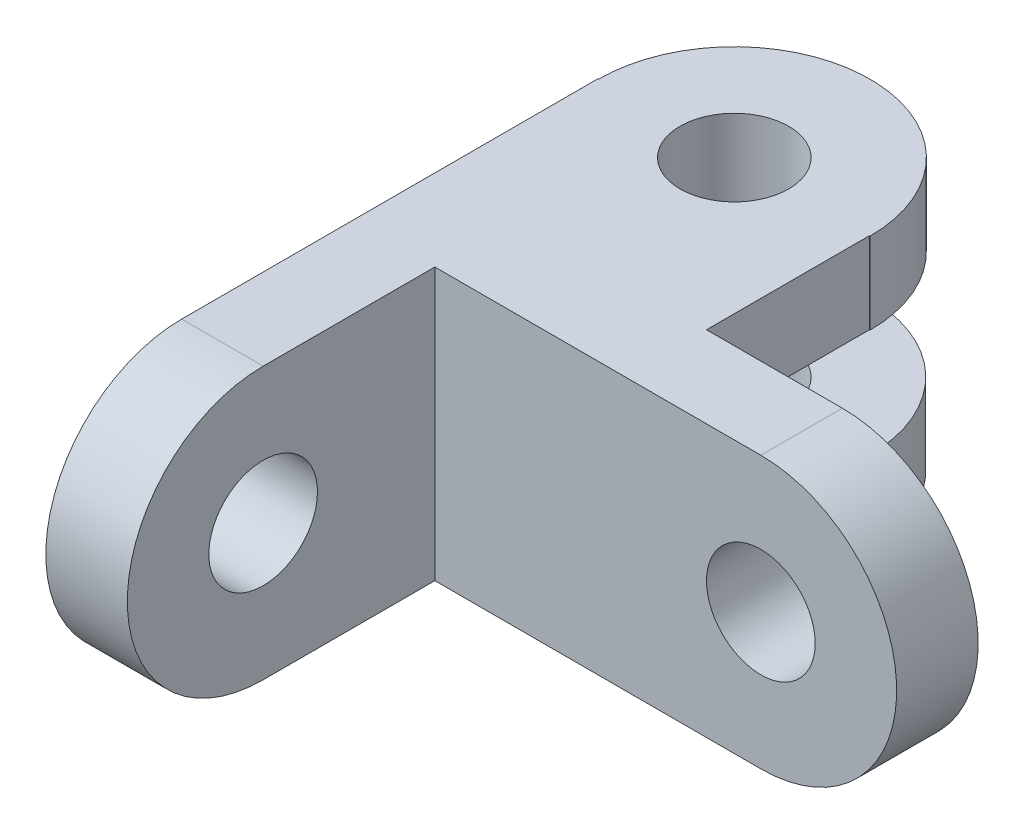
ISO-10303-21;
HEADER;
FILE_DESCRIPTION(('STEP AP214'),'2;1');
FILE_NAME('part.step','',(''),(''),'','','');
FILE_SCHEMA(('AUTOMOTIVE_DESIGN { 1 0 10303 214 1 1 1 1 }'));
ENDSEC;
DATA;
#1=APPLICATION_CONTEXT('core data for automotive mechanical design processes');
#2=APPLICATION_PROTOCOL_DEFINITION('international standard','automotive_design',2000,#1);
#3=PRODUCT_CONTEXT('',#1,'mechanical');
#4=PRODUCT('Part','Part','',(#3));
#5=PRODUCT_RELATED_PRODUCT_CATEGORY('part','',(#4));
#6=PRODUCT_DEFINITION_FORMATION('','',#4);
#7=PRODUCT_DEFINITION_CONTEXT('part definition',#1,'design');
#8=PRODUCT_DEFINITION('design','',#6,#7);
#9=PRODUCT_DEFINITION_SHAPE('','',#8);
#10=(LENGTH_UNIT() NAMED_UNIT(*) SI_UNIT(.MILLI.,.METRE.));
#11=(NAMED_UNIT(*) PLANE_ANGLE_UNIT() SI_UNIT($,.RADIAN.));
#12=(NAMED_UNIT(*) SI_UNIT($,.STERADIAN.) SOLID_ANGLE_UNIT());
#13=UNCERTAINTY_MEASURE_WITH_UNIT(LENGTH_MEASURE(1.E-05),#10,'distance_accuracy_value','');
#14=(GEOMETRIC_REPRESENTATION_CONTEXT(3) GLOBAL_UNCERTAINTY_ASSIGNED_CONTEXT((#13)) GLOBAL_UNIT_ASSIGNED_CONTEXT((#10,
#11,#12)) REPRESENTATION_CONTEXT('',''));
#15=CARTESIAN_POINT('',(0.,0.,0.));
#16=DIRECTION('',(0.,0.,1.));
#17=DIRECTION('',(1.,0.,0.));
#18=AXIS2_PLACEMENT_3D('',#15,#16,#17);
#19=CARTESIAN_POINT('',(0.,0.,6.));
#20=DIRECTION('',(0.,0.,1.));
#21=DIRECTION('',(1.,0.,0.));
#22=AXIS2_PLACEMENT_3D('',#19,#20,#21);
#23=PLANE('',#22);
#24=CARTESIAN_POINT('',(60.,20.,6.));
#25=DIRECTION('',(0.,0.,1.));
#26=DIRECTION('',(1.,0.,0.));
#27=AXIS2_PLACEMENT_3D('',#24,#25,#26);
#28=CIRCLE('',#27,8.00000000000001);
#29=CARTESIAN_POINT('',(68.,20.,6.));
#30=VERTEX_POINT('',#29);
#31=EDGE_CURVE('E519',#30,#30,#28,.T.);
#32=ORIENTED_EDGE('',*,*,#31,.F.);
#33=EDGE_LOOP('',(#32));
#34=FACE_BOUND('',#33,.T.);
#35=DIRECTION('',(1.,0.,0.));
#36=VECTOR('',#35,1.);
#37=CARTESIAN_POINT('',(0.,40.,6.));
#38=LINE('',#37,#36);
#39=CARTESIAN_POINT('',(12.,40.,6.));
#40=VERTEX_POINT('',#39);
#41=CARTESIAN_POINT('',(60.,40.,6.));
#42=VERTEX_POINT('',#41);
#43=EDGE_CURVE('E252',#40,#42,#38,.T.);
#44=ORIENTED_EDGE('',*,*,#43,.F.);
#45=DIRECTION('',(0.,-1.,0.));
#46=VECTOR('',#45,1.);
#47=CARTESIAN_POINT('',(12.,40.,6.));
#48=LINE('',#47,#46);
#49=CARTESIAN_POINT('',(12.,0.,6.));
#50=VERTEX_POINT('',#49);
#51=EDGE_CURVE('E161',#40,#50,#48,.T.);
#52=ORIENTED_EDGE('',*,*,#51,.T.);
#53=DIRECTION('',(1.,0.,0.));
#54=VECTOR('',#53,1.);
#55=CARTESIAN_POINT('',(0.,0.,6.));
#56=LINE('',#55,#54);
#57=CARTESIAN_POINT('',(60.,0.,6.));
#58=VERTEX_POINT('',#57);
#59=EDGE_CURVE('E162',#50,#58,#56,.T.);
#60=ORIENTED_EDGE('',*,*,#59,.T.);
#61=CARTESIAN_POINT('',(60.,20.,6.));
#62=DIRECTION('',(0.,0.,1.));
#63=DIRECTION('',(1.,0.,0.));
#64=AXIS2_PLACEMENT_3D('',#61,#62,#63);
#65=CIRCLE('',#64,20.);
#66=EDGE_CURVE('E250',#58,#42,#65,.T.);
#67=ORIENTED_EDGE('',*,*,#66,.T.);
#68=EDGE_LOOP('',(#44,#52,#60,#67));
#69=FACE_BOUND('',#68,.T.);
#70=ADVANCED_FACE('F41',(#34,#69),#23,.T.);
#71=CARTESIAN_POINT('',(0.,0.,-6.));
#72=DIRECTION('',(0.,0.,1.));
#73=DIRECTION('',(1.,0.,0.));
#74=AXIS2_PLACEMENT_3D('',#71,#72,#73);
#75=PLANE('',#74);
#76=CARTESIAN_POINT('',(60.,20.,-6.));
#77=DIRECTION('',(0.,0.,1.));
#78=DIRECTION('',(1.,0.,0.));
#79=AXIS2_PLACEMENT_3D('',#76,#77,#78);
#80=CIRCLE('',#79,8.00000000000001);
#81=CARTESIAN_POINT('',(68.,20.,-6.));
#82=VERTEX_POINT('',#81);
#83=EDGE_CURVE('E44',#82,#82,#80,.T.);
#84=ORIENTED_EDGE('',*,*,#83,.T.);
#85=EDGE_LOOP('',(#84));
#86=FACE_BOUND('',#85,.T.);
#87=DIRECTION('',(1.,0.,0.));
#88=VECTOR('',#87,1.);
#89=CARTESIAN_POINT('',(0.,28.,-6.));
#90=LINE('',#89,#88);
#91=CARTESIAN_POINT('',(0.,28.,-6.));
#92=VERTEX_POINT('',#91);
#93=CARTESIAN_POINT('',(40.,28.,-6.));
#94=VERTEX_POINT('',#93);
#95=EDGE_CURVE('E69',#92,#94,#90,.T.);
#96=ORIENTED_EDGE('',*,*,#95,.T.);
#97=DIRECTION('',(0.,1.,0.));
#98=VECTOR('',#97,1.);
#99=CARTESIAN_POINT('',(40.,28.,-6.));
#100=LINE('',#99,#98);
#101=CARTESIAN_POINT('',(40.,40.,-6.));
#102=VERTEX_POINT('',#101);
#103=EDGE_CURVE('E197',#94,#102,#100,.T.);
#104=ORIENTED_EDGE('',*,*,#103,.T.);
#105=DIRECTION('',(1.,0.,0.));
#106=VECTOR('',#105,1.);
#107=CARTESIAN_POINT('',(0.,40.,-6.));
#108=LINE('',#107,#106);
#109=CARTESIAN_POINT('',(60.,40.,-6.));
#110=VERTEX_POINT('',#109);
#111=EDGE_CURVE('E259',#102,#110,#108,.T.);
#112=ORIENTED_EDGE('',*,*,#111,.T.);
#113=CARTESIAN_POINT('',(60.,20.,-6.));
#114=DIRECTION('',(0.,0.,1.));
#115=DIRECTION('',(1.,0.,0.));
#116=AXIS2_PLACEMENT_3D('',#113,#114,#115);
#117=CIRCLE('',#116,20.);
#118=CARTESIAN_POINT('',(60.,0.,-6.));
#119=VERTEX_POINT('',#118);
#120=EDGE_CURVE('E253',#119,#110,#117,.T.);
#121=ORIENTED_EDGE('',*,*,#120,.F.);
#122=DIRECTION('',(1.,0.,0.));
#123=VECTOR('',#122,1.);
#124=CARTESIAN_POINT('',(0.,0.,-6.));
#125=LINE('',#124,#123);
#126=CARTESIAN_POINT('',(40.,0.,-6.00000000000001));
#127=VERTEX_POINT('',#126);
#128=EDGE_CURVE('E241',#127,#119,#125,.T.);
#129=ORIENTED_EDGE('',*,*,#128,.F.);
#130=DIRECTION('',(0.,1.,0.));
#131=VECTOR('',#130,1.);
#132=CARTESIAN_POINT('',(40.,0.,-6.00000000000001));
#133=LINE('',#132,#131);
#134=CARTESIAN_POINT('',(40.,12.,-6.00000000000001));
#135=VERTEX_POINT('',#134);
#136=EDGE_CURVE('E230',#127,#135,#133,.T.);
#137=ORIENTED_EDGE('',*,*,#136,.T.);
#138=DIRECTION('',(1.,0.,0.));
#139=VECTOR('',#138,1.);
#140=CARTESIAN_POINT('',(0.,12.,-6.));
#141=LINE('',#140,#139);
#142=CARTESIAN_POINT('',(0.,12.,-6.));
#143=VERTEX_POINT('',#142);
#144=EDGE_CURVE('E211',#143,#135,#141,.T.);
#145=ORIENTED_EDGE('',*,*,#144,.F.);
#146=DIRECTION('',(0.,1.,0.));
#147=VECTOR('',#146,1.);
#148=CARTESIAN_POINT('',(0.,0.,-6.));
#149=LINE('',#148,#147);
#150=EDGE_CURVE('E247',#143,#92,#149,.T.);
#151=ORIENTED_EDGE('',*,*,#150,.T.);
#152=EDGE_LOOP('',(#96,#104,#112,#121,#129,#137,#145,#151));
#153=FACE_BOUND('',#152,.T.);
#154=ADVANCED_FACE('F282',(#86,#153),#75,.F.);
#155=CARTESIAN_POINT('',(0.,0.,6.));
#156=DIRECTION('',(0.,1.,0.));
#157=DIRECTION('',(0.,0.,1.));
#158=AXIS2_PLACEMENT_3D('',#155,#156,#157);
#159=PLANE('',#158);
#160=CARTESIAN_POINT('',(20.0952694716515,0.,-30.));
#161=DIRECTION('',(0.,1.,0.));
#162=DIRECTION('',(0.,0.,1.));
#163=AXIS2_PLACEMENT_3D('',#160,#161,#162);
#164=CIRCLE('',#163,8.);
#165=CARTESIAN_POINT('',(20.0952694716515,0.,-22.));
#166=VERTEX_POINT('',#165);
#167=EDGE_CURVE('E173',#166,#166,#164,.T.);
#168=ORIENTED_EDGE('',*,*,#167,.T.);
#169=EDGE_LOOP('',(#168));
#170=FACE_BOUND('',#169,.T.);
#171=DIRECTION('',(0.,0.,-1.));
#172=VECTOR('',#171,1.);
#173=CARTESIAN_POINT('',(0.,0.,6.));
#174=LINE('',#173,#172);
#175=CARTESIAN_POINT('',(0.,0.,31.2796315767416));
#176=VERTEX_POINT('',#175);
#177=CARTESIAN_POINT('',(0.,0.,-30.));
#178=VERTEX_POINT('',#177);
#179=EDGE_CURVE('E254',#176,#178,#174,.T.);
#180=ORIENTED_EDGE('',*,*,#179,.T.);
#181=CARTESIAN_POINT('',(20.,0.,-30.));
#182=DIRECTION('',(0.,1.,0.));
#183=DIRECTION('',(0.,0.,1.));
#184=AXIS2_PLACEMENT_3D('',#181,#182,#183);
#185=CIRCLE('',#184,20.);
#186=CARTESIAN_POINT('',(40.,0.,-30.));
#187=VERTEX_POINT('',#186);
#188=EDGE_CURVE('E221',#187,#178,#185,.T.);
#189=ORIENTED_EDGE('',*,*,#188,.F.);
#190=DIRECTION('',(0.,0.,-1.));
#191=VECTOR('',#190,1.);
#192=CARTESIAN_POINT('',(40.,0.,-6.00000000000001));
#193=LINE('',#192,#191);
#194=EDGE_CURVE('E224',#127,#187,#193,.T.);
#195=ORIENTED_EDGE('',*,*,#194,.F.);
#196=ORIENTED_EDGE('',*,*,#128,.T.);
#197=DIRECTION('',(0.,0.,-1.));
#198=VECTOR('',#197,1.);
#199=CARTESIAN_POINT('',(60.,0.,6.));
#200=LINE('',#199,#198);
#201=EDGE_CURVE('E11',#58,#119,#200,.T.);
#202=ORIENTED_EDGE('',*,*,#201,.F.);
#203=ORIENTED_EDGE('',*,*,#59,.F.);
#204=DIRECTION('',(0.,0.,1.));
#205=VECTOR('',#204,1.);
#206=CARTESIAN_POINT('',(12.,0.,6.00000000000001));
#207=LINE('',#206,#205);
#208=CARTESIAN_POINT('',(12.,0.,31.2796315767416));
#209=VERTEX_POINT('',#208);
#210=EDGE_CURVE('E59',#50,#209,#207,.T.);
#211=ORIENTED_EDGE('',*,*,#210,.T.);
#212=DIRECTION('',(-1.,0.,0.));
#213=VECTOR('',#212,1.);
#214=CARTESIAN_POINT('',(12.,0.,31.2796315767416));
#215=LINE('',#214,#213);
#216=EDGE_CURVE('E147',#209,#176,#215,.T.);
#217=ORIENTED_EDGE('',*,*,#216,.T.);
#218=EDGE_LOOP('',(#180,#189,#195,#196,#202,#203,#211,#217));
#219=FACE_BOUND('',#218,.T.);
#220=ADVANCED_FACE('F43',(#170,#219),#159,.F.);
#221=CARTESIAN_POINT('',(60.,20.,6.));
#222=DIRECTION('',(0.,0.,-1.));
#223=DIRECTION('',(-1.,0.,0.));
#224=AXIS2_PLACEMENT_3D('',#221,#222,#223);
#225=CYLINDRICAL_SURFACE('',#224,20.);
#226=ORIENTED_EDGE('',*,*,#120,.T.);
#227=DIRECTION('',(0.,0.,-1.));
#228=VECTOR('',#227,1.);
#229=CARTESIAN_POINT('',(60.,40.,6.));
#230=LINE('',#229,#228);
#231=EDGE_CURVE('E49',#42,#110,#230,.T.);
#232=ORIENTED_EDGE('',*,*,#231,.F.);
#233=ORIENTED_EDGE('',*,*,#66,.F.);
#234=ORIENTED_EDGE('',*,*,#201,.T.);
#235=EDGE_LOOP('',(#226,#232,#233,#234));
#236=FACE_BOUND('',#235,.T.);
#237=ADVANCED_FACE('F310',(#236),#225,.T.);
#238=CARTESIAN_POINT('',(0.,40.,6.));
#239=DIRECTION('',(0.,1.,0.));
#240=DIRECTION('',(0.,0.,1.));
#241=AXIS2_PLACEMENT_3D('',#238,#239,#240);
#242=PLANE('',#241);
#243=CARTESIAN_POINT('',(20.0952694716515,40.,-30.));
#244=DIRECTION('',(0.,1.,0.));
#245=DIRECTION('',(0.,0.,1.));
#246=AXIS2_PLACEMENT_3D('',#243,#244,#245);
#247=CIRCLE('',#246,8.);
#248=CARTESIAN_POINT('',(20.0952694716515,40.,-22.));
#249=VERTEX_POINT('',#248);
#250=EDGE_CURVE('E171',#249,#249,#247,.T.);
#251=ORIENTED_EDGE('',*,*,#250,.F.);
#252=EDGE_LOOP('',(#251));
#253=FACE_BOUND('',#252,.T.);
#254=ORIENTED_EDGE('',*,*,#111,.F.);
#255=DIRECTION('',(0.,0.,-1.));
#256=VECTOR('',#255,1.);
#257=CARTESIAN_POINT('',(40.,40.,-6.));
#258=LINE('',#257,#256);
#259=CARTESIAN_POINT('',(40.,40.,-30.));
#260=VERTEX_POINT('',#259);
#261=EDGE_CURVE('E185',#102,#260,#258,.T.);
#262=ORIENTED_EDGE('',*,*,#261,.T.);
#263=DIRECTION('',(1.,0.,0.));
#264=VECTOR('',#263,1.);
#265=CARTESIAN_POINT('',(40.0952694716515,40.,-30.));
#266=LINE('',#265,#264);
#267=CARTESIAN_POINT('',(40.0952694716515,40.,-30.));
#268=VERTEX_POINT('',#267);
#269=EDGE_CURVE('E202',#260,#268,#266,.T.);
#270=ORIENTED_EDGE('',*,*,#269,.T.);
#271=CARTESIAN_POINT('',(20.0952694716515,40.,-30.));
#272=DIRECTION('',(0.,1.,0.));
#273=DIRECTION('',(0.,0.,1.));
#274=AXIS2_PLACEMENT_3D('',#271,#272,#273);
#275=CIRCLE('',#274,20.);
#276=CARTESIAN_POINT('',(0.095269471651456,40.,-30.));
#277=VERTEX_POINT('',#276);
#278=EDGE_CURVE('E207',#268,#277,#275,.T.);
#279=ORIENTED_EDGE('',*,*,#278,.T.);
#280=DIRECTION('',(-1.,0.,0.));
#281=VECTOR('',#280,1.);
#282=CARTESIAN_POINT('',(0.,40.,-30.));
#283=LINE('',#282,#281);
#284=CARTESIAN_POINT('',(0.,40.,-30.));
#285=VERTEX_POINT('',#284);
#286=EDGE_CURVE('E187',#277,#285,#283,.T.);
#287=ORIENTED_EDGE('',*,*,#286,.T.);
#288=DIRECTION('',(0.,0.,-1.));
#289=VECTOR('',#288,1.);
#290=CARTESIAN_POINT('',(0.,40.,6.));
#291=LINE('',#290,#289);
#292=CARTESIAN_POINT('',(0.,40.,31.2796315767416));
#293=VERTEX_POINT('',#292);
#294=EDGE_CURVE('E261',#293,#285,#291,.T.);
#295=ORIENTED_EDGE('',*,*,#294,.F.);
#296=DIRECTION('',(-1.,0.,0.));
#297=VECTOR('',#296,1.);
#298=CARTESIAN_POINT('',(12.,40.,31.2796315767416));
#299=LINE('',#298,#297);
#300=CARTESIAN_POINT('',(12.,40.,31.2796315767416));
#301=VERTEX_POINT('',#300);
#302=EDGE_CURVE('E153',#301,#293,#299,.T.);
#303=ORIENTED_EDGE('',*,*,#302,.F.);
#304=DIRECTION('',(0.,0.,-1.));
#305=VECTOR('',#304,1.);
#306=CARTESIAN_POINT('',(12.,40.,6.));
#307=LINE('',#306,#305);
#308=EDGE_CURVE('E152',#301,#40,#307,.T.);
#309=ORIENTED_EDGE('',*,*,#308,.T.);
#310=ORIENTED_EDGE('',*,*,#43,.T.);
#311=ORIENTED_EDGE('',*,*,#231,.T.);
#312=EDGE_LOOP('',(#254,#262,#270,#279,#287,#295,#303,#309,#310,#311));
#313=FACE_BOUND('',#312,.T.);
#314=ADVANCED_FACE('F302',(#253,#313),#242,.T.);
#315=CARTESIAN_POINT('',(0.,0.,6.));
#316=DIRECTION('',(-1.,0.,0.));
#317=DIRECTION('',(0.,0.,1.));
#318=AXIS2_PLACEMENT_3D('',#315,#316,#317);
#319=PLANE('',#318);
#320=CARTESIAN_POINT('',(0.,20.,31.2796315767416));
#321=DIRECTION('',(1.,0.,0.));
#322=DIRECTION('',(0.,0.,-1.));
#323=AXIS2_PLACEMENT_3D('',#320,#321,#322);
#324=CIRCLE('',#323,8.);
#325=CARTESIAN_POINT('',(0.,20.,23.2796315767416));
#326=VERTEX_POINT('',#325);
#327=EDGE_CURVE('E167',#326,#326,#324,.T.);
#328=ORIENTED_EDGE('',*,*,#327,.T.);
#329=EDGE_LOOP('',(#328));
#330=FACE_BOUND('',#329,.T.);
#331=ORIENTED_EDGE('',*,*,#150,.F.);
#332=DIRECTION('',(0.,0.,-1.));
#333=VECTOR('',#332,1.);
#334=CARTESIAN_POINT('',(0.,12.,-6.));
#335=LINE('',#334,#333);
#336=CARTESIAN_POINT('',(0.,12.,-30.));
#337=VERTEX_POINT('',#336);
#338=EDGE_CURVE('E228',#143,#337,#335,.T.);
#339=ORIENTED_EDGE('',*,*,#338,.T.);
#340=DIRECTION('',(0.,1.,0.));
#341=VECTOR('',#340,1.);
#342=CARTESIAN_POINT('',(0.,0.,-30.));
#343=LINE('',#342,#341);
#344=EDGE_CURVE('E237',#178,#337,#343,.T.);
#345=ORIENTED_EDGE('',*,*,#344,.F.);
#346=ORIENTED_EDGE('',*,*,#179,.F.);
#347=CARTESIAN_POINT('',(0.,20.,31.2796315767416));
#348=DIRECTION('',(-1.,0.,0.));
#349=DIRECTION('',(0.,0.,1.));
#350=AXIS2_PLACEMENT_3D('',#347,#348,#349);
#351=CIRCLE('',#350,20.);
#352=EDGE_CURVE('E151',#176,#293,#351,.T.);
#353=ORIENTED_EDGE('',*,*,#352,.T.);
#354=ORIENTED_EDGE('',*,*,#294,.T.);
#355=DIRECTION('',(0.,1.,0.));
#356=VECTOR('',#355,1.);
#357=CARTESIAN_POINT('',(0.,28.,-30.));
#358=LINE('',#357,#356);
#359=CARTESIAN_POINT('',(0.,28.,-30.));
#360=VERTEX_POINT('',#359);
#361=EDGE_CURVE('E212',#360,#285,#358,.T.);
#362=ORIENTED_EDGE('',*,*,#361,.F.);
#363=DIRECTION('',(0.,0.,1.));
#364=VECTOR('',#363,1.);
#365=CARTESIAN_POINT('',(0.,28.,-6.));
#366=LINE('',#365,#364);
#367=EDGE_CURVE('E182',#360,#92,#366,.T.);
#368=ORIENTED_EDGE('',*,*,#367,.T.);
#369=EDGE_LOOP('',(#331,#339,#345,#346,#353,#354,#362,#368));
#370=FACE_BOUND('',#369,.T.);
#371=ADVANCED_FACE('F297',(#330,#370),#319,.T.);
#372=CARTESIAN_POINT('',(20.,0.,-30.));
#373=DIRECTION('',(0.,1.,0.));
#374=DIRECTION('',(0.,0.,1.));
#375=AXIS2_PLACEMENT_3D('',#372,#373,#374);
#376=CYLINDRICAL_SURFACE('',#375,20.);
#377=CARTESIAN_POINT('',(20.,12.,-30.));
#378=DIRECTION('',(0.,1.,0.));
#379=DIRECTION('',(0.,0.,1.));
#380=AXIS2_PLACEMENT_3D('',#377,#378,#379);
#381=CIRCLE('',#380,20.);
#382=CARTESIAN_POINT('',(40.,12.,-30.));
#383=VERTEX_POINT('',#382);
#384=EDGE_CURVE('E234',#383,#337,#381,.T.);
#385=ORIENTED_EDGE('',*,*,#384,.F.);
#386=DIRECTION('',(0.,1.,0.));
#387=VECTOR('',#386,1.);
#388=CARTESIAN_POINT('',(40.,0.,-30.));
#389=LINE('',#388,#387);
#390=EDGE_CURVE('E245',#187,#383,#389,.T.);
#391=ORIENTED_EDGE('',*,*,#390,.F.);
#392=ORIENTED_EDGE('',*,*,#188,.T.);
#393=ORIENTED_EDGE('',*,*,#344,.T.);
#394=EDGE_LOOP('',(#385,#391,#392,#393));
#395=FACE_BOUND('',#394,.T.);
#396=ADVANCED_FACE('F303',(#395),#376,.T.);
#397=CARTESIAN_POINT('',(40.,0.,-6.00000000000001));
#398=DIRECTION('',(1.,0.,0.));
#399=DIRECTION('',(0.,0.,-1.));
#400=AXIS2_PLACEMENT_3D('',#397,#398,#399);
#401=PLANE('',#400);
#402=DIRECTION('',(0.,0.,-1.));
#403=VECTOR('',#402,1.);
#404=CARTESIAN_POINT('',(40.,12.,-6.00000000000001));
#405=LINE('',#404,#403);
#406=EDGE_CURVE('E233',#135,#383,#405,.T.);
#407=ORIENTED_EDGE('',*,*,#406,.F.);
#408=ORIENTED_EDGE('',*,*,#136,.F.);
#409=ORIENTED_EDGE('',*,*,#194,.T.);
#410=ORIENTED_EDGE('',*,*,#390,.T.);
#411=EDGE_LOOP('',(#407,#408,#409,#410));
#412=FACE_BOUND('',#411,.T.);
#413=ADVANCED_FACE('F300',(#412),#401,.T.);
#414=CARTESIAN_POINT('',(20.,12.,-30.));
#415=DIRECTION('',(0.,1.,0.));
#416=DIRECTION('',(0.,0.,1.));
#417=AXIS2_PLACEMENT_3D('',#414,#415,#416);
#418=PLANE('',#417);
#419=CARTESIAN_POINT('',(20.0952694716515,12.,-30.));
#420=DIRECTION('',(0.,1.,0.));
#421=DIRECTION('',(0.,0.,1.));
#422=AXIS2_PLACEMENT_3D('',#419,#420,#421);
#423=CIRCLE('',#422,8.);
#424=CARTESIAN_POINT('',(20.0952694716515,12.,-22.));
#425=VERTEX_POINT('',#424);
#426=EDGE_CURVE('E177',#425,#425,#423,.T.);
#427=ORIENTED_EDGE('',*,*,#426,.F.);
#428=EDGE_LOOP('',(#427));
#429=FACE_BOUND('',#428,.T.);
#430=ORIENTED_EDGE('',*,*,#144,.T.);
#431=ORIENTED_EDGE('',*,*,#406,.T.);
#432=ORIENTED_EDGE('',*,*,#384,.T.);
#433=ORIENTED_EDGE('',*,*,#338,.F.);
#434=EDGE_LOOP('',(#430,#431,#432,#433));
#435=FACE_BOUND('',#434,.T.);
#436=ADVANCED_FACE('F347',(#429,#435),#418,.T.);
#437=CARTESIAN_POINT('',(0.,28.,-30.));
#438=DIRECTION('',(0.,0.,-1.));
#439=DIRECTION('',(-1.,0.,0.));
#440=AXIS2_PLACEMENT_3D('',#437,#438,#439);
#441=PLANE('',#440);
#442=ORIENTED_EDGE('',*,*,#286,.F.);
#443=DIRECTION('',(0.,1.,0.));
#444=VECTOR('',#443,1.);
#445=CARTESIAN_POINT('',(0.095269471651456,28.,-30.));
#446=LINE('',#445,#444);
#447=CARTESIAN_POINT('',(0.095269471651456,28.,-30.));
#448=VERTEX_POINT('',#447);
#449=EDGE_CURVE('E213',#448,#277,#446,.T.);
#450=ORIENTED_EDGE('',*,*,#449,.F.);
#451=DIRECTION('',(-1.,0.,0.));
#452=VECTOR('',#451,1.);
#453=CARTESIAN_POINT('',(0.,28.,-30.));
#454=LINE('',#453,#452);
#455=EDGE_CURVE('E196',#448,#360,#454,.T.);
#456=ORIENTED_EDGE('',*,*,#455,.T.);
#457=ORIENTED_EDGE('',*,*,#361,.T.);
#458=EDGE_LOOP('',(#442,#450,#456,#457));
#459=FACE_BOUND('',#458,.T.);
#460=ADVANCED_FACE('F338',(#459),#441,.T.);
#461=CARTESIAN_POINT('',(20.0952694716515,28.,-30.));
#462=DIRECTION('',(0.,1.,0.));
#463=DIRECTION('',(0.,0.,1.));
#464=AXIS2_PLACEMENT_3D('',#461,#462,#463);
#465=CYLINDRICAL_SURFACE('',#464,20.);
#466=ORIENTED_EDGE('',*,*,#278,.F.);
#467=DIRECTION('',(0.,1.,0.));
#468=VECTOR('',#467,1.);
#469=CARTESIAN_POINT('',(40.0952694716515,28.,-30.));
#470=LINE('',#469,#468);
#471=CARTESIAN_POINT('',(40.0952694716515,28.,-30.));
#472=VERTEX_POINT('',#471);
#473=EDGE_CURVE('E216',#472,#268,#470,.T.);
#474=ORIENTED_EDGE('',*,*,#473,.F.);
#475=CARTESIAN_POINT('',(20.0952694716515,28.,-30.));
#476=DIRECTION('',(0.,1.,0.));
#477=DIRECTION('',(0.,0.,1.));
#478=AXIS2_PLACEMENT_3D('',#475,#476,#477);
#479=CIRCLE('',#478,20.);
#480=EDGE_CURVE('E191',#472,#448,#479,.T.);
#481=ORIENTED_EDGE('',*,*,#480,.T.);
#482=ORIENTED_EDGE('',*,*,#449,.T.);
#483=EDGE_LOOP('',(#466,#474,#481,#482));
#484=FACE_BOUND('',#483,.T.);
#485=ADVANCED_FACE('F344',(#484),#465,.T.);
#486=CARTESIAN_POINT('',(40.0952694716515,28.,-30.));
#487=DIRECTION('',(0.,0.,1.));
#488=DIRECTION('',(1.,0.,0.));
#489=AXIS2_PLACEMENT_3D('',#486,#487,#488);
#490=PLANE('',#489);
#491=ORIENTED_EDGE('',*,*,#269,.F.);
#492=DIRECTION('',(0.,1.,0.));
#493=VECTOR('',#492,1.);
#494=CARTESIAN_POINT('',(40.,28.,-30.));
#495=LINE('',#494,#493);
#496=CARTESIAN_POINT('',(40.,28.,-30.));
#497=VERTEX_POINT('',#496);
#498=EDGE_CURVE('E218',#497,#260,#495,.T.);
#499=ORIENTED_EDGE('',*,*,#498,.F.);
#500=DIRECTION('',(1.,0.,0.));
#501=VECTOR('',#500,1.);
#502=CARTESIAN_POINT('',(40.0952694716515,28.,-30.));
#503=LINE('',#502,#501);
#504=EDGE_CURVE('E192',#497,#472,#503,.T.);
#505=ORIENTED_EDGE('',*,*,#504,.T.);
#506=ORIENTED_EDGE('',*,*,#473,.T.);
#507=EDGE_LOOP('',(#491,#499,#505,#506));
#508=FACE_BOUND('',#507,.T.);
#509=ADVANCED_FACE('F346',(#508),#490,.T.);
#510=CARTESIAN_POINT('',(40.,28.,-6.));
#511=DIRECTION('',(1.,0.,0.));
#512=DIRECTION('',(0.,0.,-1.));
#513=AXIS2_PLACEMENT_3D('',#510,#511,#512);
#514=PLANE('',#513);
#515=ORIENTED_EDGE('',*,*,#261,.F.);
#516=ORIENTED_EDGE('',*,*,#103,.F.);
#517=DIRECTION('',(0.,0.,-1.));
#518=VECTOR('',#517,1.);
#519=CARTESIAN_POINT('',(40.,28.,-6.));
#520=LINE('',#519,#518);
#521=EDGE_CURVE('E189',#94,#497,#520,.T.);
#522=ORIENTED_EDGE('',*,*,#521,.T.);
#523=ORIENTED_EDGE('',*,*,#498,.T.);
#524=EDGE_LOOP('',(#515,#516,#522,#523));
#525=FACE_BOUND('',#524,.T.);
#526=ADVANCED_FACE('F284',(#525),#514,.T.);
#527=CARTESIAN_POINT('',(20.0952694716515,28.,-30.));
#528=DIRECTION('',(0.,1.,0.));
#529=DIRECTION('',(0.,0.,1.));
#530=AXIS2_PLACEMENT_3D('',#527,#528,#529);
#531=PLANE('',#530);
#532=CARTESIAN_POINT('',(20.0952694716515,28.,-30.));
#533=DIRECTION('',(0.,1.,0.));
#534=DIRECTION('',(0.,0.,1.));
#535=AXIS2_PLACEMENT_3D('',#532,#533,#534);
#536=CIRCLE('',#535,8.);
#537=CARTESIAN_POINT('',(20.0952694716515,28.,-22.));
#538=VERTEX_POINT('',#537);
#539=EDGE_CURVE('E176',#538,#538,#536,.T.);
#540=ORIENTED_EDGE('',*,*,#539,.T.);
#541=EDGE_LOOP('',(#540));
#542=FACE_BOUND('',#541,.T.);
#543=ORIENTED_EDGE('',*,*,#367,.F.);
#544=ORIENTED_EDGE('',*,*,#455,.F.);
#545=ORIENTED_EDGE('',*,*,#480,.F.);
#546=ORIENTED_EDGE('',*,*,#504,.F.);
#547=ORIENTED_EDGE('',*,*,#521,.F.);
#548=ORIENTED_EDGE('',*,*,#95,.F.);
#549=EDGE_LOOP('',(#543,#544,#545,#546,#547,#548));
#550=FACE_BOUND('',#549,.T.);
#551=ADVANCED_FACE('F267',(#542,#550),#531,.F.);
#552=CARTESIAN_POINT('',(20.0952694716515,0.,-30.));
#553=DIRECTION('',(0.,1.,0.));
#554=DIRECTION('',(0.,0.,1.));
#555=AXIS2_PLACEMENT_3D('',#552,#553,#554);
#556=CYLINDRICAL_SURFACE('',#555,8.);
#557=ORIENTED_EDGE('',*,*,#250,.T.);
#558=EDGE_LOOP('',(#557));
#559=FACE_BOUND('',#558,.T.);
#560=ORIENTED_EDGE('',*,*,#539,.F.);
#561=EDGE_LOOP('',(#560));
#562=FACE_BOUND('',#561,.T.);
#563=ADVANCED_FACE('F272',(#559,#562),#556,.F.);
#564=ORIENTED_EDGE('',*,*,#426,.T.);
#565=EDGE_LOOP('',(#564));
#566=FACE_BOUND('',#565,.T.);
#567=ORIENTED_EDGE('',*,*,#167,.F.);
#568=EDGE_LOOP('',(#567));
#569=FACE_BOUND('',#568,.T.);
#570=ADVANCED_FACE('F271',(#566,#569),#556,.F.);
#571=CARTESIAN_POINT('',(12.,20.,31.2796315767416));
#572=DIRECTION('',(-1.,0.,0.));
#573=DIRECTION('',(0.,0.,1.));
#574=AXIS2_PLACEMENT_3D('',#571,#572,#573);
#575=CYLINDRICAL_SURFACE('',#574,20.);
#576=ORIENTED_EDGE('',*,*,#352,.F.);
#577=ORIENTED_EDGE('',*,*,#216,.F.);
#578=CARTESIAN_POINT('',(12.,20.,31.2796315767416));
#579=DIRECTION('',(-1.,0.,0.));
#580=DIRECTION('',(0.,0.,1.));
#581=AXIS2_PLACEMENT_3D('',#578,#579,#580);
#582=CIRCLE('',#581,20.);
#583=EDGE_CURVE('E146',#209,#301,#582,.T.);
#584=ORIENTED_EDGE('',*,*,#583,.T.);
#585=ORIENTED_EDGE('',*,*,#302,.T.);
#586=EDGE_LOOP('',(#576,#577,#584,#585));
#587=FACE_BOUND('',#586,.T.);
#588=ADVANCED_FACE('F150',(#587),#575,.T.);
#589=CARTESIAN_POINT('',(12.,20.,31.2796315767416));
#590=DIRECTION('',(-1.,0.,0.));
#591=DIRECTION('',(0.,0.,1.));
#592=AXIS2_PLACEMENT_3D('',#589,#590,#591);
#593=PLANE('',#592);
#594=CARTESIAN_POINT('',(12.,20.,31.2796315767416));
#595=DIRECTION('',(1.,0.,0.));
#596=DIRECTION('',(0.,0.,-1.));
#597=AXIS2_PLACEMENT_3D('',#594,#595,#596);
#598=CIRCLE('',#597,8.);
#599=CARTESIAN_POINT('',(12.,20.,23.2796315767416));
#600=VERTEX_POINT('',#599);
#601=EDGE_CURVE('E524',#600,#600,#598,.T.);
#602=ORIENTED_EDGE('',*,*,#601,.F.);
#603=EDGE_LOOP('',(#602));
#604=FACE_BOUND('',#603,.T.);
#605=ORIENTED_EDGE('',*,*,#51,.F.);
#606=ORIENTED_EDGE('',*,*,#308,.F.);
#607=ORIENTED_EDGE('',*,*,#583,.F.);
#608=ORIENTED_EDGE('',*,*,#210,.F.);
#609=EDGE_LOOP('',(#605,#606,#607,#608));
#610=FACE_BOUND('',#609,.T.);
#611=ADVANCED_FACE('F159',(#604,#610),#593,.F.);
#612=CARTESIAN_POINT('',(0.,20.,31.2796315767416));
#613=DIRECTION('',(1.,0.,0.));
#614=DIRECTION('',(0.,0.,-1.));
#615=AXIS2_PLACEMENT_3D('',#612,#613,#614);
#616=CYLINDRICAL_SURFACE('',#615,8.);
#617=ORIENTED_EDGE('',*,*,#327,.F.);
#618=EDGE_LOOP('',(#617));
#619=FACE_BOUND('',#618,.T.);
#620=ORIENTED_EDGE('',*,*,#601,.T.);
#621=EDGE_LOOP('',(#620));
#622=FACE_BOUND('',#621,.T.);
#623=ADVANCED_FACE('F453',(#619,#622),#616,.F.);
#624=CARTESIAN_POINT('',(60.,20.,-50.));
#625=DIRECTION('',(0.,0.,1.));
#626=DIRECTION('',(1.,0.,0.));
#627=AXIS2_PLACEMENT_3D('',#624,#625,#626);
#628=CYLINDRICAL_SURFACE('',#627,8.00000000000001);
#629=ORIENTED_EDGE('',*,*,#31,.T.);
#630=EDGE_LOOP('',(#629));
#631=FACE_BOUND('',#630,.T.);
#632=ORIENTED_EDGE('',*,*,#83,.F.);
#633=EDGE_LOOP('',(#632));
#634=FACE_BOUND('',#633,.T.);
#635=ADVANCED_FACE('F465',(#631,#634),#628,.F.);
#636=CLOSED_SHELL('',(#70,#154,#220,#237,#314,#371,#396,#413,#436,#460,#485,#509,#526,#551,#563,
#570,#588,#611,#623,#635));
#637=MANIFOLD_SOLID_BREP('B2',#636);
#638=ADVANCED_BREP_SHAPE_REPRESENTATION('',(#18,#637),#14);
#639=SHAPE_DEFINITION_REPRESENTATION(#9,#638);
ENDSEC;
END-ISO-10303-21;
